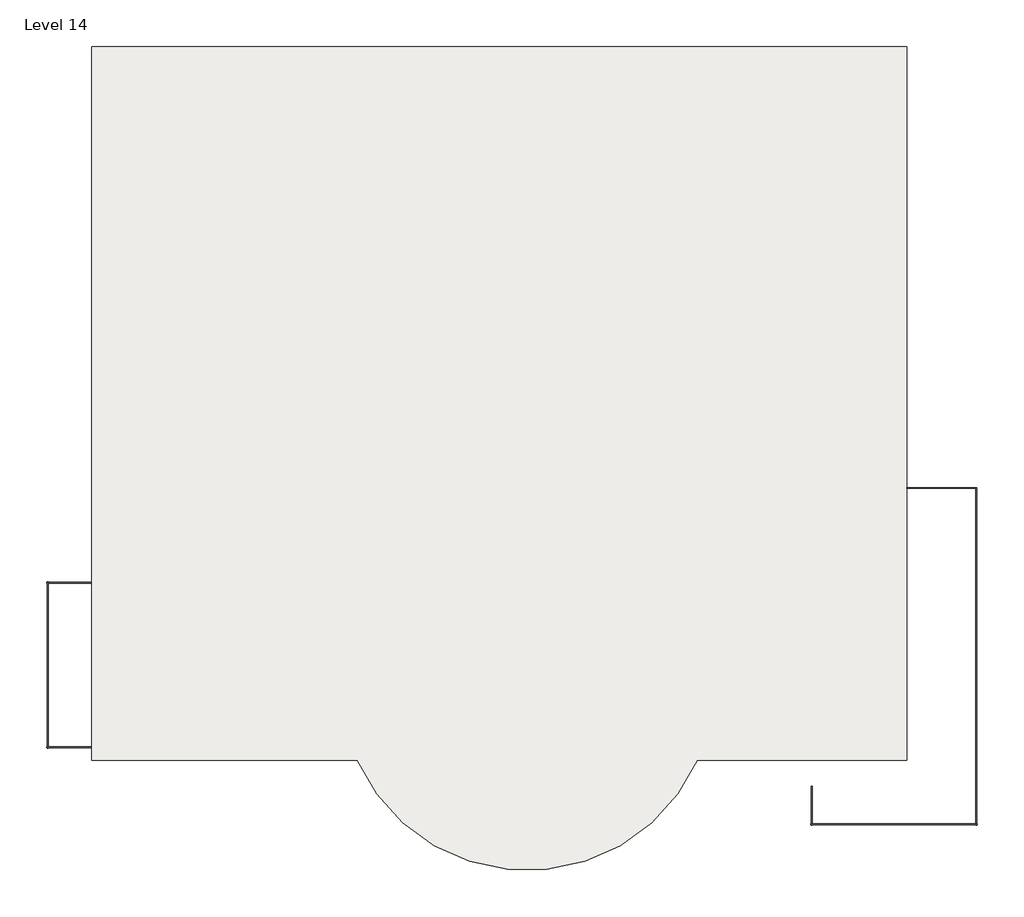
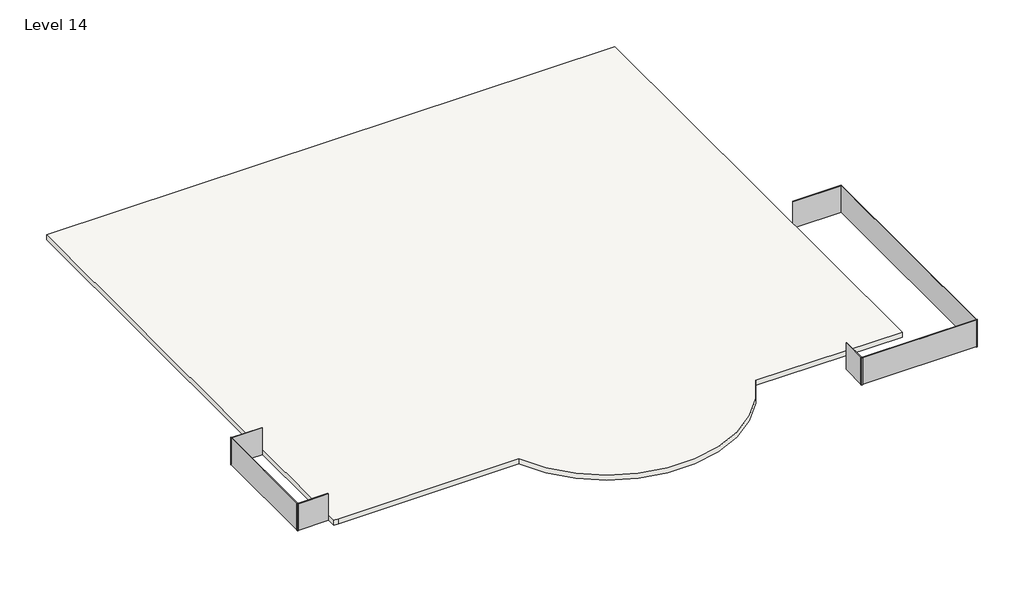
# One storey: 7 plates, 1 slab.
"""IFC4 building model written with IfcOpenShell, lengths in millimetres."""

from ifc_helpers import new_model, si_unit, point, frame, frame_2d, origin, place, context, project, spatial, polyline, circle_curve, trimmed, segment, composite_curve, outline, extrude, transform, mapped, element, save
from components import system_panel_glazed_7d767388, system_panel_glazed_c55d8a5b, system_panel_glazed_4fcd3a06, system_panel_glazed_e4a816a2, system_panel_glazed_019fba88

model = new_model("IFC4")

# Units and contexts
model_context = context("Model", 3, world=origin())
ifc_project = project(units=[si_unit("LENGTHUNIT", "METRE", prefix="MILLI")], contexts=[model_context])

# Site, building, storey
site = spatial("IfcSite", under=ifc_project)
building = spatial("IfcBuilding", under=site)
storey = spatial("IfcBuildingStorey", under=building, Name="Level 14", Elevation=22707.6)

# Plates
placement = place(None, origin())
system_panel_glazed_shape = system_panel_glazed_7d767388(model_context)
element("IfcPlate", 1, ObjectType="System Panel : Glazed", at=placement, inside=storey, context=model_context, shape_type="MappedRepresentation", body=[
    mapped(system_panel_glazed_shape, transform((-17306.4505427, -8690.0239591, 22707.6), x_axis=(-1.0, 0.0, 0.0), y_axis=(0.0, -1.0, 0.0), z_axis=(0.0, 0.0, 1.0))),
])
element("IfcPlate", 2, ObjectType="System Panel : Glazed", at=placement, inside=storey, context=model_context, shape_type="MappedRepresentation", body=[
    mapped(system_panel_glazed_shape, transform((-17306.4505427, -13719.2239591, 22707.6), x_axis=(1.0, 0.0, 0.0), y_axis=(0.0, 1.0, 0.0), z_axis=(0.0, 0.0, 1.0))),
])
system_panel_glazed_2_shape = system_panel_glazed_c55d8a5b(model_context)
element("IfcPlate", 3, ObjectType="System Panel : Glazed", at=placement, inside=storey, context=model_context, shape_type="MappedRepresentation", body=[
    mapped(system_panel_glazed_2_shape, transform((-17979.5505427, -11204.6239591, 22707.6), x_axis=(0.0, -1.0, 0.0), y_axis=(1.0, 0.0, 0.0), z_axis=(0.0, 0.0, 1.0))),
])
element("IfcPlate", 4, ObjectType="System Panel : Glazed", at=placement, inside=storey, context=model_context, shape_type="MappedRepresentation", body=[
    mapped(system_panel_glazed_2_shape, transform((7603.0464352, -16040.2308221, 22707.6), x_axis=(1.0, 0.0, 0.0), y_axis=(0.0, 1.0, 0.0), z_axis=(0.0, 0.0, 1.0))),
])
system_panel_glazed_3_shape = system_panel_glazed_4fcd3a06(model_context)
element("IfcPlate", 5, ObjectType="System Panel : Glazed", at=placement, inside=storey, context=model_context, shape_type="MappedRepresentation", body=[
    mapped(system_panel_glazed_3_shape, transform((9031.7964352, -5892.9308221, 22707.6), x_axis=(1.0, 0.0, 0.0), y_axis=(0.0, 1.0, 0.0), z_axis=(0.0, 0.0, 1.0))),
])
system_panel_glazed_4_shape = system_panel_glazed_e4a816a2(model_context)
element("IfcPlate", 6, ObjectType="System Panel : Glazed", at=placement, inside=storey, context=model_context, shape_type="MappedRepresentation", body=[
    mapped(system_panel_glazed_4_shape, transform((5088.4464352, -15449.2043258, 22707.6), x_axis=(0.0, -1.0, 0.0), y_axis=(1.0, 0.0, 0.0), z_axis=(0.0, 0.0, 1.0))),
])
system_panel_glazed_5_shape = system_panel_glazed_019fba88(model_context)
element("IfcPlate", 7, ObjectType="System Panel : Glazed", at=placement, inside=storey, context=model_context, shape_type="MappedRepresentation", body=[
    mapped(system_panel_glazed_5_shape, transform((10117.6464352, -10944.3558221, 22707.6), x_axis=(0.0, 1.0, 0.0), y_axis=(-1.0, 0.0, 0.0), z_axis=(0.0, 0.0, 1.0))),
])

# Slab
element("IfcSlab", 8, ObjectType="9\"", at=placement, inside=storey, context=model_context, shape_type="SweptSolid", body=[
    extrude(outline(composite_curve([segment(polyline([(-16607.9505427, 7461.1191779), (7979.2494573, 7461.1191779), (7979.2494573, -14078.0808221), (1652.8739931, -14078.0808221)]), True, "CONTINUOUS"), segment(trimmed(circle_curve(frame_2d((-3476.1505427, -11788.3650223)), 5616.9111737), [point((1652.8739931, -14078.0808221))], [point((-8605.1750786, -14078.0808221))], False, "CARTESIAN"), True, "CONTINUOUS"), segment(polyline([(-8605.1750786, -14078.0808221), (-16404.7505427, -14078.0808221), (-16607.9505427, -14078.0808221), (-16607.9505427, 7461.1191779)]), True, "CONTINUOUS")], self_intersect=False)), frame((0.0, 0.0, 22707.6), z_axis=(0.0, 0.0, 1.0), x_axis=(1.0, 0.0, 0.0)), (0.0, 0.0, 1.0), 228.6),
])

save(model, "model.ifc")

# Revit data of these elements
# Type "System Panel : Glazed"
#   Construction Type Id = "GSP4R"
#   Analytic Construction = "1/8 in Pilkington single glazing"
#   Visual Light Transmittance = 0.9
#   Solar Heat Gain Coefficient = 0.86
#   Heat Transfer Coefficient (U) = 1.18115 BTU/(h·ft²·°F)
# Type "9\""
#   Assembly Code = "B1010"
#   Function = 0
#   Layers, outside or top first: 0' - 9" no material (function 1)
# Elements 1, 2, 3, 4, 5, 6, 7 (IfcPlate, "System Panel : Glazed")
#   Phase Created = New Construction
#   Materials on its faces: "Glass"
# Element 8 (IfcSlab, "9\"")
#   built-in parameter 1001955 = 1.5708 (stored number, unit not read)
#   Height Offset From Level = 0' - 9"
#   Phase Created = New Construction
#   Materials on its faces: "Default Floor"
# Materials
#   "Glass": class "Glass", colour RGB 0 128 192, transparency 0.75, Description = "Soda Lime Glass", Cost = 0
#   "Default Floor": colour RGB 128 128 128, transparency 0
